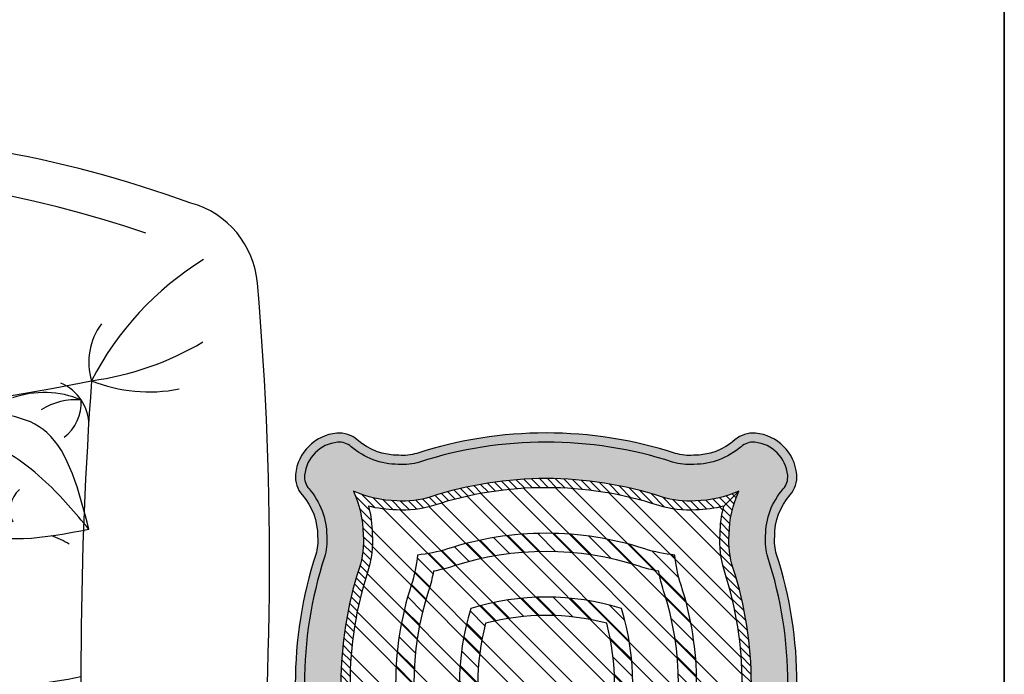
# Model space of a CAD drawing. Units: inches. Extents: x 844 to 2234, y 346 to 1084.
# Tile 41 of 93: x 1266.41 to 1283.62, y 719.22 to 730.66. Entities that reach past the tile are written whole.
import ezdxf

# ---------------------------------------------------------------- set-up
doc = ezdxf.new("R2010")
doc.units = ezdxf.units.IN
doc.header["$MEASUREMENT"] = 0
doc.layers.add('A-WALL', color=7, linetype='Continuous', lineweight=35)
doc.layers.add('furniture', color=8, linetype='Continuous', lineweight=18)
for name, color, linetype in [('RA-AP-01$0$FURN', 3, 'Continuous'), ('RA-AP-01$0$steel', 193, 'Continuous'), ('RA-AP-01$0$WOOD', 64, 'Continuous')]:
    doc.layers.add(name, color=color, linetype=linetype)
pattern_1 = [(45, (0, 1.362436106329781), (-0.0088388347648318, 0.0088388347648318), [])]
pattern_2 = [(45, (0, 1.362436106329781), (-0.0044194173824159, 0.0044194173824159), [])]

# ---------------------------------------------------------------- blocks, each defined once
blk = doc.blocks.new('A$C2FCF5309')
at = {"layer": 'RA-AP-01$0$FURN'}
h = blk.add_hatch(dxfattribs=at)
h.set_pattern_fill('ANSI31', color=256, scale=0.1, style=0)
h.set_pattern_definition(pattern_1)
h.paths.add_polyline_path([(5.038683893313746, -5.169250834004607, -0.1583983521602212), (5.038683893312098, -5.373464580902012, 0.0306258898943267), (5.033304057242972, -5.394827569605182, 0.0306258898948892), (5.01194106853941, -5.40020740567441, -0.1028142994996694), (4.878286182323899, -5.414871334512708), (4.863600873530158, -5.43331743520547, 0.1120482678681049), (5.018059823131753, -5.419248541734471, -0.052642197802937), (5.050972078299936, -5.412495590662115, -0.0526421977994963), (5.057725029371615, -5.379583335496025, 0.1583028414702701), (5.057725029372958, -5.163132079409654, -0.052642197806903), (5.050972078299777, -5.130219824239078, -0.0526421977995126), (5.018059823133679, -5.123466873167369, 0.0215995840215353), (4.988903013548211, -5.115372132362452), (4.975007495303644, -5.132826183367946, -0.0289147572844802), (5.011941068537408, -5.142508009226167, 0.0306258898976746), (5.033304057242868, -5.147887845296027, 0.0306258899022411)])
h.paths.add_polyline_path([(4.975007495303645, -5.132826183367946), (4.988903013548211, -5.115372132362452, 0.1362374241599938), (4.801608567045604, -5.12346687316654, -0.0526421978036853), (4.768696311876971, -5.130219824239102, -0.05264219780204), (4.761943360804856, -5.163132079406747, 0.1583028414743723), (4.761943360806116, -5.379583335498449, -0.0526421977955461), (4.768696311877141, -5.412495590662114, -0.0526421978073986), (4.801608567048022, -5.419248541735437, 0.0454484293938888), (4.863600873530158, -5.43331743520547), (4.878286182323899, -5.414871334512708, -0.0546933379798044), (4.80772732164382, -5.40020740567649, 0.030625889903973), (4.786364332934043, -5.394827569605216, 0.0306258898932853), (4.780984496865101, -5.373464580902791, -0.1583983521638281), (4.780984496864308, -5.169250834000963, 0.03062588989692), (4.786364332933943, -5.147887845296004, 0.0306258898946324), (4.807727321637318, -5.142508009226805, -0.1288932573266927)])
h.paths.add_polyline_path([(4.843422214712861, -5.204945727074827, -0.0783685831716868), (4.924134454130224, -5.196727409635105), (4.939146578618322, -5.177870798323143, 0.1012675676854134), (4.827248748758957, -5.188772261120899, 0.1253648873081696), (4.820394258584192, -5.327034652050361), (4.837127701354095, -5.306015906404253, -0.0981593964869636)], flags=17)
h.paths.add_polyline_path([(4.843422214712824, -5.337769687826355, -0.0311091841722656), (4.837127701354095, -5.306015906404253), (4.820394258584193, -5.32703465205036, 0.0247727657431944), (4.827248748758908, -5.353943153780261, 0.0812754385032542), (4.916962478476905, -5.36629034358622), (4.933684093813825, -5.345286454285511, -0.0876255421014372)], flags=17)
h.paths.add_polyline_path([(4.992419641418037, -5.353943153780226, 0.1506053783834298), (4.992419641417933, -5.188772261120954, 0.0485966419124224), (4.939146578618321, -5.177870798323143), (4.924134454130224, -5.196727409635105, -0.0507799419579301), (4.976246175464031, -5.204945727074882, -0.1296645318906876), (4.97624617546411, -5.337769687826316, -0.0415667119298777), (4.933684093813825, -5.345286454285511), (4.916962478476905, -5.36629034358622, 0.0684915676023693)], flags=17)
h = blk.add_hatch(dxfattribs=at)
h.set_pattern_fill('ANSI31', color=256, scale=0.1, style=0)
h.set_pattern_definition(pattern_1)
h.paths.add_polyline_path([(5.038683893313746, -5.169250834004607, -0.1583983521602212), (5.038683893312098, -5.373464580902012, 0.0306258898943267), (5.033304057242972, -5.394827569605182, 0.0306258898948892), (5.01194106853941, -5.40020740567441, -0.1028142994996694), (4.878286182323899, -5.414871334512708), (4.863600873530158, -5.43331743520547, 0.1120482678681049), (5.018059823131753, -5.419248541734471, -0.052642197802937), (5.050972078299936, -5.412495590662115, -0.0526421977994963), (5.057725029371615, -5.379583335496025, 0.1583028414702701), (5.057725029372958, -5.163132079409654, -0.052642197806903), (5.050972078299777, -5.130219824239078, -0.0526421977995126), (5.018059823133679, -5.123466873167369, 0.0215995840215353), (4.988903013548211, -5.115372132362452), (4.975007495303644, -5.132826183367946, -0.0289147572844802), (5.011941068537408, -5.142508009226167, 0.0306258898976746), (5.033304057242868, -5.147887845296027, 0.0306258899022411)])
h.paths.add_polyline_path([(4.975007495303645, -5.132826183367946), (4.988903013548211, -5.115372132362452, 0.1362374241599938), (4.801608567045604, -5.12346687316654, -0.0526421978036853), (4.768696311876971, -5.130219824239102, -0.05264219780204), (4.761943360804856, -5.163132079406747, 0.1583028414743723), (4.761943360806116, -5.379583335498449, -0.0526421977955461), (4.768696311877141, -5.412495590662114, -0.0526421978073986), (4.801608567048022, -5.419248541735437, 0.0454484293938888), (4.863600873530158, -5.43331743520547), (4.878286182323899, -5.414871334512708, -0.0546933379798044), (4.80772732164382, -5.40020740567649, 0.030625889903973), (4.786364332934043, -5.394827569605216, 0.0306258898932853), (4.780984496865101, -5.373464580902791, -0.1583983521638281), (4.780984496864308, -5.169250834000963, 0.03062588989692), (4.786364332933943, -5.147887845296004, 0.0306258898946324), (4.807727321637318, -5.142508009226805, -0.1288932573266927)])
h.paths.add_polyline_path([(4.843422214712861, -5.204945727074827, -0.0783685831716868), (4.924134454130224, -5.196727409635105), (4.939146578618322, -5.177870798323143, 0.1012675676854134), (4.827248748758957, -5.188772261120899, 0.1253648873081696), (4.820394258584192, -5.327034652050361), (4.837127701354095, -5.306015906404253, -0.0981593964869636)], flags=17)
h.paths.add_polyline_path([(4.843422214712824, -5.337769687826355, -0.0311091841722656), (4.837127701354095, -5.306015906404253), (4.820394258584193, -5.32703465205036, 0.0247727657431944), (4.827248748758908, -5.353943153780261, 0.0812754385032542), (4.916962478476905, -5.36629034358622), (4.933684093813825, -5.345286454285511, -0.0876255421014372)], flags=17)
h.paths.add_polyline_path([(4.992419641418037, -5.353943153780226, 0.1506053783834298), (4.992419641417933, -5.188772261120954, 0.0485966419124224), (4.939146578618321, -5.177870798323143), (4.924134454130224, -5.196727409635105, -0.0507799419579301), (4.976246175464031, -5.204945727074882, -0.1296645318906876), (4.97624617546411, -5.337769687826316, -0.0415667119298777), (4.933684093813825, -5.345286454285511), (4.916962478476905, -5.36629034358622, 0.0684915676023693)], flags=17)
at = {"layer": 'RA-AP-01$0$WOOD'}
h = blk.add_hatch(color=256, dxfattribs=at)
edge = h.paths.add_edge_path()
edge.add_arc((4.683001772622394, -5.026441828662609), 0.0299999999999998, 48.77105092035535, 95.25687599427813)
edge.add_arc((4.684834195088484, -5.046357707450686), 0.0499999999998897, 95.25687599443106, 174.7431240064049)
edge.add_arc((4.664918316300367, -5.044525284985046), 0.0300000000000005, 174.7431240062535, 221.2289490796905)
edge.add_arc((4.591236830209155, -5.109094338216345), 0.0679700159630267, -0.5333070513215148, 41.228949079691915, ccw=False)
edge.add_arc((4.609451302807284, -5.114694777173187), 0.0500000000000008, -17.3556839752095, 5.7020707654044145, ccw=False)
edge.add_arc((5.095208119646659, -5.271357707450659), 0.4603971832811796, 162.0683908477609, 197.9316091523306)
edge.add_arc((4.609451302807533, -5.428020637728902), 0.0500000000000006, -5.702070765320514, 17.355683975293914, ccw=False)
edge.add_arc((4.591236830209412, -5.433621076685779), 0.0679700159630261, -41.228949079600625, 0.5333070514128053, ccw=False)
edge.add_arc((4.664918316300727, -5.498190129916959), 0.0299999999999995, 138.7710509204022, 185.256875994324)
edge.add_arc((4.684834195088642, -5.496357707450695), 0.0499999999997451, 185.2568759946742, 264.74312400432)
edge.add_arc((4.683001772622394, -5.516273586238612), 0.03, 264.743124003969, 311.2289490796446)
edge.add_arc((4.747570825853633, -5.589955072329876), 0.0679700159630271, 89.4666929486321, 131.2289490796457, ccw=False)
edge.add_arc((4.753171264810493, -5.57174059973175), 0.0500000000000015, 72.64431602474701, 95.70207076536133, ccw=False)
edge.add_arc((4.909834195088355, -5.085983782892503), 0.4603971832811774, 252.0683908477147, 287.9316091522845)
edge.add_arc((5.06649712536621, -5.57174059973175), 0.0499999999999999, 84.29792923463953, 107.35568397525361, ccw=False)
edge.add_arc((5.072097564323069, -5.589955072329877), 0.0679700159630274, 48.771050920354185, 90.5333070513679, ccw=False)
edge.add_arc((5.136666617554309, -5.516273586238614), 0.0299999999999997, 228.771050920353, 275.2568759942969)
edge.add_arc((5.134834195088338, -5.496357707450417), 0.0499999999999982, 275.2568759942949, 354.7431240057633)
edge.add_arc((5.154750073876535, -5.498190129916372), 0.0299999999999999, 354.7431240057662, 401.2289490796891)
edge.add_arc((5.228431559967749, -5.433621076685074), 0.0679700159630274, 179.4666929486771, 221.2289490796903, ccw=False)
edge.add_arc((5.210217087369615, -5.428020637728227), 0.0499999999999976, 162.6443160247947, 185.7020707654089, ccw=False)
edge.add_arc((4.724460270530244, -5.271357707450757), 0.4603971832811793, 342.0683908477607, 377.9316091523305)
edge.add_arc((5.210217087369368, -5.114694777172509), 0.0500000000000019, 174.2979292346878, 197.355683975302, ccw=False)
edge.add_arc((5.228431559967489, -5.109094338215639), 0.0679700159630279, 138.7710509203993, 180.5333070514128, ccw=False)
edge.add_arc((5.154750073876174, -5.044525284984457), 0.0300000000000001, 318.771050920401, 365.2568759954636)
edge.add_arc((5.13483419508816, -5.046357707450624), 0.0499999999998349, 5.256875995237118, 84.74312400549572)
edge.add_arc((5.136666617554308, -5.026441828662608), 0.0299999999999994, 84.74312400572185, 131.2289490796446)
edge.add_arc((5.072097564323072, -4.952760342571343), 0.0679700159630261, 269.4666929486298, 311.22894907964354, ccw=False)
edge.add_arc((5.066497125366206, -4.97097481516947), 0.0499999999999992, 252.64431602475162, 275.70207076536565, ccw=False)
edge.add_arc((4.909834195088355, -5.456731632008717), 0.4603971832811764, 72.06839084771546, 107.9316091522853)
edge.add_arc((4.753171264810493, -4.970974815169471), 0.0500000000000016, 264.2979292346387, 287.355683975253, ccw=False)
edge.add_arc((4.747570825853633, -4.952760342571346), 0.0679700159630274, 228.7710509203543, 270.5333070513679, ccw=False)
edge = h.paths.add_edge_path(flags=16)
edge.add_arc((4.683001772622395, -5.026441828662608), 0.019999999999999, 48.7710509203555, 95.2568759942793)
edge.add_arc((4.684834195088469, -5.046357707450671), 0.0399999999998731, 95.2568759944489, 174.7431240064248)
edge.add_arc((4.664918316300404, -5.044525284985035), 0.020000000000036, 174.7431240062186, 221.2289490796461)
edge.add_arc((4.591236830209151, -5.109094338216346), 0.0779700159630296, -0.13764630038667747, 41.228949079689585, ccw=False)
edge.add_arc((4.609451302807307, -5.11469477717304), 0.060000000000024, -17.406127045137907, 5.176192161068002, ccw=False)
edge.add_arc((5.09520811964665, -5.271357707450659), 0.4503971832811708, 162.0623235129628, 197.9376764869162)
edge.add_arc((4.609451302807532, -5.428020637728943), 0.0599999999999982, -5.176192160466428, 17.406127046715312, ccw=False)
edge.add_arc((4.591236830209414, -5.433621076685778), 0.0779700159630257, -41.2289490796029, 0.13764630095249686, ccw=False)
edge.add_arc((4.664918316300731, -5.498190129916961), 0.0200000000000047, 138.7710509204103, 185.2568759943212)
edge.add_arc((4.684834195088606, -5.496357707450731), 0.0399999999997066, 185.2568759947174, 264.7431240043665)
edge.add_arc((4.683001772622369, -5.516273586238541), 0.020000000000069, 264.7431240038842, 311.2289490795622)
edge.add_arc((4.747570825853635, -5.589955072329884), 0.0779700159630344, 89.8623536987642, 131.2289490796432, ccw=False)
edge.add_arc((4.753171264810603, -5.571740599731771), 0.0599999999999895, 72.5938729544394, 95.1761921602253, ccw=False)
edge.add_arc((4.909834195088365, -5.085983782892505), 0.4503971832811724, 252.0623235129989, 287.9376764870498)
edge.add_arc((5.066497125366216, -5.571740599731755), 0.0600000000000047, 84.8238078399923, 107.40612704528041, ccw=False)
edge.add_arc((5.072097564322998, -5.589955072329853), 0.077970015963056, 48.771050920303594, 90.13764630126451, ccw=False)
edge.add_arc((5.136666617554307, -5.516273586238622), 0.0199999999999931, 228.771050920344, 275.2568759943037)
edge.add_arc((5.134834195088338, -5.496357707450416), 0.0400000000000004, 275.2568759942928, 354.7431240057607)
edge.add_arc((5.154750073876533, -5.498190129916375), 0.0200000000000037, 354.7431240057783, 401.2289490796939)
edge.add_arc((5.228431559967745, -5.433621076685076), 0.0779700159630239, 179.8623536995147, 221.2289490796908, ccw=False)
edge.add_arc((5.210217087369586, -5.428020637728345), 0.0600000000000054, 162.5938729554486, 185.1761921609759, ccw=False)
edge.add_arc((4.724460270530243, -5.271357707450766), 0.4503971832811826, 342.0623235128896, 377.937676486982)
edge.add_arc((5.210217087369347, -5.114694777172486), 0.0599999999999777, 174.8238078387611, 197.4061270462219, ccw=False)
edge.add_arc((5.228431559967523, -5.109094338215542), 0.0779700159629885, 138.7710509204687, 180.1376463004423, ccw=False)
edge.add_arc((5.154750073876175, -5.044525284984459), 0.0199999999999989, 318.771050920406, 365.2568759954698)
edge.add_arc((5.134834195088138, -5.046357707450646), 0.0399999999998586, 5.256875995208452, 84.74312400546732)
edge.add_arc((5.136666617554292, -5.02644182866256), 0.0199999999999529, 84.74312400577769, 131.2289490797025)
edge.add_arc((5.072097564323069, -4.952760342571338), 0.077970015963032, 269.86235369901414, 311.2289490796421, ccw=False)
edge.add_arc((5.06649712536618, -4.97097481516946), 0.0600000000000007, 252.5938729548277, 275.17619216047467, ccw=False)
edge.add_arc((4.909834195088353, -5.456731632008716), 0.4503971832811739, 72.06232351293887, 107.9376764867365)
edge.add_arc((4.753171264810429, -4.970974815169467), 0.0599999999999991, 264.82380783985815, 287.40612704769893, ccw=False)
edge.add_arc((4.747570825853681, -4.952760342571361), 0.0779700159630467, 228.7710509203206, 270.13764630113724, ccw=False)
h = blk.add_hatch(color=256, dxfattribs=at)
edge = h.paths.add_edge_path()
edge.add_arc((4.683001772622395, -5.026441828662608), 0.019999999999999, 48.7710509203555, 95.2568759942793)
edge.add_arc((4.684834195088469, -5.046357707450671), 0.0399999999998731, 95.2568759944489, 174.7431240064248)
edge.add_arc((4.664918316300404, -5.044525284985035), 0.020000000000036, 174.7431240062186, 221.2289490796461)
edge.add_arc((4.591236830209151, -5.109094338216346), 0.0779700159630296, -0.13764630038667747, 41.228949079689585, ccw=False)
edge.add_arc((4.609451302807307, -5.11469477717304), 0.060000000000024, -17.406127045137907, 5.176192161068002, ccw=False)
edge.add_arc((5.09520811964665, -5.271357707450659), 0.4503971832811708, 162.0623235129628, 197.9376764869162)
edge.add_arc((4.609451302807532, -5.428020637728943), 0.0599999999999982, -5.176192160466428, 17.406127046715312, ccw=False)
edge.add_arc((4.591236830209414, -5.433621076685778), 0.0779700159630257, -41.2289490796029, 0.13764630095249686, ccw=False)
edge.add_arc((4.664918316300731, -5.498190129916961), 0.0200000000000047, 138.7710509204103, 185.2568759943212)
edge.add_arc((4.684834195088606, -5.496357707450731), 0.0399999999997066, 185.2568759947174, 264.7431240043665)
edge.add_arc((4.683001772622369, -5.516273586238541), 0.020000000000069, 264.7431240038842, 311.2289490795622)
edge.add_arc((4.747570825853635, -5.589955072329884), 0.0779700159630344, 89.8623536987642, 131.2289490796432, ccw=False)
edge.add_arc((4.753171264810603, -5.571740599731771), 0.0599999999999895, 72.5938729544394, 95.1761921602253, ccw=False)
edge.add_arc((4.909834195088365, -5.085983782892505), 0.4503971832811724, 252.0623235129989, 287.9376764870498)
edge.add_arc((5.066497125366216, -5.571740599731755), 0.0600000000000047, 84.8238078399923, 107.40612704528041, ccw=False)
edge.add_arc((5.072097564322998, -5.589955072329853), 0.077970015963056, 48.771050920303594, 90.13764630126451, ccw=False)
edge.add_arc((5.136666617554307, -5.516273586238622), 0.0199999999999931, 228.771050920344, 275.2568759943037)
edge.add_arc((5.134834195088338, -5.496357707450416), 0.0400000000000004, 275.2568759942928, 354.7431240057607)
edge.add_arc((5.154750073876533, -5.498190129916375), 0.0200000000000037, 354.7431240057783, 401.2289490796939)
edge.add_arc((5.228431559967745, -5.433621076685076), 0.0779700159630239, 179.8623536995147, 221.2289490796908, ccw=False)
edge.add_arc((5.210217087369586, -5.428020637728345), 0.0600000000000054, 162.5938729554486, 185.1761921609759, ccw=False)
edge.add_arc((4.724460270530243, -5.271357707450766), 0.4503971832811826, 342.0623235128896, 377.937676486982)
edge.add_arc((5.210217087369347, -5.114694777172486), 0.0599999999999777, 174.8238078387611, 197.4061270462219, ccw=False)
edge.add_arc((5.228431559967523, -5.109094338215542), 0.0779700159629885, 138.7710509204687, 180.1376463004423, ccw=False)
edge.add_arc((5.154750073876175, -5.044525284984459), 0.0199999999999989, 318.771050920406, 365.2568759954698)
edge.add_arc((5.134834195088138, -5.046357707450646), 0.0399999999998586, 5.256875995208452, 84.74312400546732)
edge.add_arc((5.136666617554292, -5.02644182866256), 0.0199999999999529, 84.74312400577769, 131.2289490797025)
edge.add_arc((5.072097564323069, -4.952760342571338), 0.077970015963032, 269.86235369901414, 311.2289490796421, ccw=False)
edge.add_arc((5.06649712536618, -4.97097481516946), 0.0600000000000007, 252.5938729548277, 275.17619216047467, ccw=False)
edge.add_arc((4.909834195088353, -5.456731632008716), 0.4503971832811739, 72.06232351293887, 107.9376764867365)
edge.add_arc((4.753171264810429, -4.970974815169467), 0.0599999999999991, 264.82380783985815, 287.40612704769893, ccw=False)
edge.add_arc((4.747570825853681, -4.952760342571361), 0.0779700159630467, 228.7710509203206, 270.13764630113724, ccw=False)
edge = h.paths.add_edge_path(flags=16)
edge.add_arc((4.591236830209151, -5.109094338216348), 0.1179700159630308, 0.7417751874182841, 24.563326950263672, ccw=False)
edge.add_arc((4.609451302807302, -5.114694777173093), 0.100000000000012, -17.52836504564658, 4.087328884225087, ccw=False)
edge.add_arc((5.095208119646651, -5.271357707450657), 0.4103971832811724, 162.0403002448777, 197.9596997550675)
edge.add_arc((4.60945130280753, -5.428020637728918), 0.1000000000000027, -4.087328883827581, 17.528365046291924, ccw=False)
edge.add_arc((4.591236830209414, -5.433621076685779), 0.1179700159630246, 335.43667305041845, 359.2582248129738, ccw=False)
edge.add_arc((4.747570825853596, -5.589955072329891), 0.117970015963042, 90.7417751868461, 114.5633269496104, ccw=False)
edge.add_arc((4.753171264810559, -5.571740599731767), 0.0999999999999976, 72.47163495370341, 94.0873288836737, ccw=False)
edge.add_arc((4.909834195088367, -5.085983782892503), 0.4103971832811735, 252.0403002449999, 287.9596997551833)
edge.add_arc((5.066497125366205, -5.571740599731755), 0.1000000000000057, 85.91267111645209, 107.5283650455624, ccw=False)
edge.add_arc((5.072097564322985, -5.58995507232986), 0.117970015963046, 65.4366730497672, 89.25822481317113, ccw=False)
edge.add_arc((5.22843155996773, -5.433621076684992), 0.1179700159630096, 180.7417751873964, 204.5633269502712, ccw=False)
edge.add_arc((5.210217087369591, -5.428020637728301), 0.0999999999999969, 162.4716349546276, 184.0873288841682, ccw=False)
edge.add_arc((4.724460270530243, -5.271357707450766), 0.4103971832811825, 342.0403002448147, 377.9596997550345)
edge.add_arc((5.210217087369347, -5.114694777172489), 0.0999999999999796, 175.9126711156995, 197.5283650464392, ccw=False)
edge.add_arc((5.228431559967512, -5.109094338215525), 0.1179700159630019, 155.4366730502992, 179.2582248126247, ccw=False)
edge.add_arc((5.072097564323172, -4.952760342571314), 0.1179700159630537, 270.74177518697286, 294.56332694975765, ccw=False)
edge.add_arc((5.066497125366189, -4.970974815169462), 0.1000000000000017, 252.471634954247, 274.0873288838353, ccw=False)
edge.add_arc((4.909834195088353, -5.456731632008716), 0.4103971832811758, 72.04030024486342, 107.9596997549354)
edge.add_arc((4.75317126481046, -4.970974815169467), 0.1000000000000041, 265.91267111635307, 287.5283650466103, ccw=False)
edge.add_arc((4.747570825853629, -4.952760342571342), 0.1179700159630538, 245.43667304992562, 269.2582248131125, ccw=False)
h = blk.add_hatch(dxfattribs=at)
h.set_pattern_fill('ANSI31', color=256, scale=0.05, style=0)
h.set_pattern_definition(pattern_2)
h.paths.add_polyline_path([(5.105336294329346, -5.394854099602528, 0.0940138826956367), (5.100476366643778, -5.435568764288975, 0.0606271852326483), (5.104678567100611, -5.466202079462671, 0.0606271852344644), (5.074045251925975, -5.46199987900586, 0.0940138827021426), (5.033330587236848, -5.466859806692645, -0.1305325492494615), (4.828072633169377, -5.477944178050054), (4.821119726105699, -5.486677669841435, 0.1336226599878005), (5.036379334063467, -5.476383803188216, -0.0945969211935747), (5.073624810952389, -5.471994942692536, -0.1043170707892296), (5.121137550891356, -5.48266106325342, -0.1043170707868944), (5.110471430330457, -5.435148323315565, -0.0945969211952573), (5.114860290825935, -5.397902846425963, 0.1580239521433527), (5.114860290826324, -5.144812568476775, -0.0945969212010491), (5.110471430330247, -5.10756709158498, -0.1043170707844371), (5.121137550890657, -5.060054351648168, -0.104317070786514), (5.073624810952866, -5.070720472208642, -0.0945969211958523), (5.036379334063063, -5.066331611712874, 0.1580239521426795), (4.783289056114906, -5.066331611712465, -0.0945969211985319), (4.746043579224103, -5.070720472208672, -0.1043170707882665), (4.698530839285552, -5.060054351647925, -0.1043170707867205), (4.709196959846443, -5.10756709158571, -0.094596921196788), (4.704808099350826, -5.144812568475902, 0.1580239521433127), (4.704808099350699, -5.397902846425022, -0.094596921197841), (4.709196959846712, -5.435148323315576, -0.1043170707855109), (4.698530839286393, -5.482661063252921, -0.1043170707864168), (4.746043579224162, -5.471994942692571, -0.0945969211977586), (4.783289056114671, -5.476383803188671, 0.0238966994662183), (4.821119726105699, -5.486677669841435), (4.828072633169378, -5.477944178050054, -0.0269814195959459), (4.786337802940177, -5.466859806692736, 0.0940138827039629), (4.745623138250268, -5.461999879005895, 0.0606271852320776), (4.714989823076826, -5.466202079462476, 0.0606271852304618), (4.719192023533341, -5.435568764289856, 0.0940138826917763), (4.714332095848404, -5.394854099604977, -0.1580706864542086), (4.714332095846561, -5.147861315302034, 0.0940138827032017), (4.719192023533127, -5.107146650612438, 0.0606271852329446), (4.714989823076289, -5.076513335438588, 0.0606271852340035), (4.745623138250698, -5.08071553589536, 0.0940138827025969), (4.786337802940015, -5.075855608208526, -0.1580706864508517), (5.033330587237968, -5.075855608208939, 0.0940138827009578), (5.074045251926627, -5.080715535895319, 0.0606271852322557), (5.104678567100159, -5.076513335438697, 0.0606271852308743), (5.100476366643561, -5.107146650611519, 0.0940138827178109), (5.105336294331983, -5.147861315307182, -0.1580706864490946)])
h = blk.add_hatch(dxfattribs=at)
h.set_pattern_fill('ANSI31', color=256, scale=0.05, style=0)
h.set_pattern_definition(pattern_2)
h.paths.add_polyline_path([(5.105336294329346, -5.394854099602528, 0.0940138826956367), (5.100476366643778, -5.435568764288975, 0.0606271852326483), (5.104678567100611, -5.466202079462671, 0.0606271852344644), (5.074045251925975, -5.46199987900586, 0.0940138827021426), (5.033330587236848, -5.466859806692645, -0.1305325492494615), (4.828072633169377, -5.477944178050054), (4.821119726105699, -5.486677669841435, 0.1336226599878005), (5.036379334063467, -5.476383803188216, -0.0945969211935747), (5.073624810952389, -5.471994942692536, -0.1043170707892296), (5.121137550891356, -5.48266106325342, -0.1043170707868944), (5.110471430330457, -5.435148323315565, -0.0945969211952573), (5.114860290825935, -5.397902846425963, 0.1580239521433527), (5.114860290826324, -5.144812568476775, -0.0945969212010491), (5.110471430330247, -5.10756709158498, -0.1043170707844371), (5.121137550890657, -5.060054351648168, -0.104317070786514), (5.073624810952866, -5.070720472208642, -0.0945969211958523), (5.036379334063063, -5.066331611712874, 0.1580239521426795), (4.783289056114906, -5.066331611712465, -0.0945969211985319), (4.746043579224103, -5.070720472208672, -0.1043170707882665), (4.698530839285552, -5.060054351647925, -0.1043170707867205), (4.709196959846443, -5.10756709158571, -0.094596921196788), (4.704808099350826, -5.144812568475902, 0.1580239521433127), (4.704808099350699, -5.397902846425022, -0.094596921197841), (4.709196959846712, -5.435148323315576, -0.1043170707855109), (4.698530839286393, -5.482661063252921, -0.1043170707864168), (4.746043579224162, -5.471994942692571, -0.0945969211977586), (4.783289056114671, -5.476383803188671, 0.0238966994662183), (4.821119726105699, -5.486677669841435), (4.828072633169378, -5.477944178050054, -0.0269814195959459), (4.786337802940177, -5.466859806692736, 0.0940138827039629), (4.745623138250268, -5.461999879005895, 0.0606271852320776), (4.714989823076826, -5.466202079462476, 0.0606271852304618), (4.719192023533341, -5.435568764289856, 0.0940138826917763), (4.714332095848404, -5.394854099604977, -0.1580706864542086), (4.714332095846561, -5.147861315302034, 0.0940138827032017), (4.719192023533127, -5.107146650612438, 0.0606271852329446), (4.714989823076289, -5.076513335438588, 0.0606271852340035), (4.745623138250698, -5.08071553589536, 0.0940138827025969), (4.786337802940015, -5.075855608208526, -0.1580706864508517), (5.033330587237968, -5.075855608208939, 0.0940138827009578), (5.074045251926627, -5.080715535895319, 0.0606271852322557), (5.104678567100159, -5.076513335438697, 0.0606271852308743), (5.100476366643561, -5.107146650611519, 0.0940138827178109), (5.105336294331983, -5.147861315307182, -0.1580706864490946)])
h = blk.add_hatch(dxfattribs=at)
h.set_pattern_fill('ANSI32,_I', color=256, scale=0.1, style=2)
h.set_pattern_definition([(45, (0, 0), (-0.0265165042944955, 0.0265165042944955), []), (45, (0.0176776695, 0), (-0.0265165042944955, 0.0265165042944955), [])])
h.paths.add_polyline_path([(4.843422214712824, -5.337769687826354, 0.1296645318905289), (4.97624617546411, -5.337769687826316, 0.1296645318906876), (4.976246175464032, -5.204945727074882, 0.129664531890418), (4.843422214712861, -5.204945727074827, 0.129664531890765)], flags=0)
h.paths.add_polyline_path([(5.039131224122924, -5.170637849998464, -0.0326520429852175), (5.033304057242868, -5.147887845296027, -0.0326520429894721), (5.010554052537512, -5.142060678415043, 0.1561383235202698), (4.809114337641437, -5.142060678414318, -0.0326520429925972), (4.786364332933944, -5.147887845296004, -0.0326520429914489), (4.780537166052582, -5.170637850002729, 0.1561383235189577), (4.780537166052134, -5.37207756489719, -0.0326520429934175), (4.786364332934042, -5.394827569605215, -0.0326520429823496), (4.809114337634529, -5.400654736484653, 0.156138323524066), (5.010554052535268, -5.400654736486903, -0.032652042992888), (5.033304057242972, -5.394827569605183, -0.0326520429928733), (5.039131224124712, -5.372077564897496, 0.1561383235226786)], flags=0)
h.paths.add_polyline_path([(4.992419641418037, -5.353943153780226, -0.1506053783832862), (4.827248748758909, -5.353943153780261, -0.1506053783835069), (4.827248748758957, -5.188772261120899, -0.1506053783831346), (4.992419641417933, -5.188772261120954, -0.1506053783834298)], flags=0)
h.paths.add_polyline_path([(4.976246175464111, -5.337769687826316, -0.1296645318905298), (4.843422214712824, -5.337769687826354, -0.129664531890765), (4.843422214712862, -5.204945727074827, -0.1296645318904162), (4.976246175464031, -5.204945727074882, -0.1296645318906876)], flags=0)
h.paths.add_polyline_path([(5.105721254232479, -5.149054940982025, -0.0968902512052664), (5.100476366643561, -5.107146650611519, -0.0606271852308743), (5.104678567100159, -5.076513335438697, -0.0606271852322574), (5.074045251926626, -5.080715535895319, -0.0968902512197216), (5.032136961550132, -5.075470648304253, 0.1564657949319774), (4.787531428625239, -5.075470648304682, -0.0968902512150626), (4.745623138250699, -5.08071553589536, -0.060627185234009), (4.714989823076288, -5.076513335438587, -0.0606271852329501), (4.719192023533127, -5.10714665061244, -0.0968902512185585), (4.713947135942331, -5.149054940988458, 0.1564657949285579), (4.713947135940853, -5.393660473908259, -0.0968902512319826), (4.71919202353334, -5.435568764289873, -0.0606271852304288), (4.714989823076825, -5.466202079462476, -0.0606271852320811), (4.745623138250269, -5.461999879005895, -0.0968902512162649), (4.787531428625332, -5.467244766596559, 0.1564657949327057), (5.032136961551311, -5.46724476659659, -0.0968902512153659), (5.074045251925975, -5.46199987900586, -0.0606271852344627), (5.10467856710061, -5.466202079462671, -0.0606271852326483), (5.100476366643777, -5.435568764288975, -0.0968902512258216), (5.105721254235559, -5.393660473909953, 0.1564657949340142)])
h.paths.add_polyline_path([(5.057725029371625, -5.379583335495999, 0.0526421977995391), (5.050972078299936, -5.412495590662114, 0.0526421978029782), (5.018059823131728, -5.419248541734479, -0.1583028414681072), (4.801608567048168, -5.419248541735485, 0.0526421978076402), (4.76869631187714, -5.412495590662113, 0.0526421977956189), (4.761943360806101, -5.379583335498404, -0.1583028414743129), (4.761943360804846, -5.163132079406778, 0.0526421978020944), (4.768696311876972, -5.130219824239101, 0.0526421978033651), (4.80160856704541, -5.123466873166602, -0.1583028414716875), (5.018059823133628, -5.123466873167353, 0.0526421977995944), (5.050972078299776, -5.130219824239078, 0.0526421978070423), (5.057725029372986, -5.163132079409739, -0.1583028414701848)], flags=16)
h.paths.add_polyline_path([(5.038683893312112, -5.373464580901968, 0.0306258898943915), (5.033304057242972, -5.394827569605182, 0.0306258898948892), (5.01194106853941, -5.40020740567441, -0.1583983521587032), (4.807727321643864, -5.400207405676503, 0.0306258899040366), (4.786364332934043, -5.394827569605215, 0.0306258898931986), (4.780984496865119, -5.37346458090285, -0.1583983521638542), (4.7809844968643, -5.169250834000989, 0.0306258898969596), (4.786364332933945, -5.147887845296004, 0.0306258898946195), (4.807727321637311, -5.142508009226808, -0.1583983521623412), (5.011941068537318, -5.142508009226139, 0.030625889897807), (5.033304057242868, -5.147887845296028, 0.0306258899020632), (5.038683893313706, -5.169250834004486, -0.1583983521602835)], flags=0)
for p, q in [((4.714989823076289, -5.076513335438588), (4.698530839285552, -5.060054351647925)), ((4.714989823076289, -5.076513335438588), (4.698530839285552, -5.060054351647925)), ((5.104678567100159, -5.076513335438697), (5.121137550890656, -5.060054351648169)), ((5.104678567100159, -5.076513335438697), (5.121137550890656, -5.060054351648169)), ((5.10467856710061, -5.466202079462671), (5.121137550891355, -5.482661063253419)), ((5.10467856710061, -5.466202079462671), (5.121137550891355, -5.482661063253419))]:
    blk.add_line(p, q, dxfattribs=at)
for points in [[(4.702773858784635, -5.003879368495489, 0.2056608120285223), (4.680253138923443, -4.996568010480312, 0.3614336704708569), (4.635044498118043, -5.041776651286372, 0.2056608120263112), (4.642355856133262, -5.064297371147306, -0.1842662638101064), (4.65920390179375, -5.10972699154053, -0.1009492694051416), (4.657174869772992, -5.129609908955028, 0.1577727036674954), (4.657174869773219, -5.41310550594699, -0.1009492694051416), (4.659203901794006, -5.432988423361486, -0.1842662638101064), (4.64235585613359, -5.478418043754737, 0.2056608120285221), (4.635044498118431, -5.500938763615934, 0.3614336704593693), (4.680253138922529, -5.546147404420826, 0.2056608120364936), (4.702773858784635, -5.538836046405732, -0.1842662638101064), (4.748203479177874, -5.52198800074528, -0.1009492694051415), (4.768086396592371, -5.524017032766053, 0.1577727036674954), (5.051581993584332, -5.524017032766055, -0.1009492694051416), (5.071464910998829, -5.521988000745282, -0.1842662638101064), (5.116894531392067, -5.538836046405734, 0.2056608120286145), (5.13941525125327, -5.546147404420911, 0.3614336704683636), (5.184623892058835, -5.500938763615299, 0.2056608120285223), (5.177312534043641, -5.478418043754112, -0.1842662638101063), (5.160464488383153, -5.432988423360887, -0.1009492694051416), (5.162493520403909, -5.41310550594639, 0.1577727036674954), (5.162493520403684, -5.129609908954428, -0.1009492694051416), (5.160464488382894, -5.109726991539933, -0.1842662638101064), (5.17731253404331, -5.064297371146681, 0.2056608120337072), (5.184623892058415, -5.041776651284888, 0.3614336704623863), (5.139415251253259, -4.99656801048031, 0.2056608120285223), (5.116894531392067, -5.003879368495487, -0.1842662638101064), (5.071464910998829, -5.020727414155937, -0.1009492694051416), (5.051581993584332, -5.018698382135166, 0.1577727036674956), (4.768086396592371, -5.018698382135168, -0.1009492694051416), (4.748203479177874, -5.020727414155941, -0.1842662638101064)], [(4.702773858784635, -5.003879368495489, 0.2056608120285223), (4.680253138923443, -4.996568010480312, 0.3614336704708569), (4.635044498118043, -5.041776651286372, 0.2056608120263112), (4.642355856133262, -5.064297371147306, -0.1842662638101064), (4.65920390179375, -5.10972699154053, -0.1009492694051416), (4.657174869772992, -5.129609908955028, 0.1577727036674954), (4.657174869773219, -5.41310550594699, -0.1009492694051416), (4.659203901794006, -5.432988423361486, -0.1842662638101064), (4.64235585613359, -5.478418043754737, 0.2056608120285221), (4.635044498118431, -5.500938763615934, 0.3614336704593693), (4.680253138922529, -5.546147404420826, 0.2056608120364936), (4.702773858784635, -5.538836046405732, -0.1842662638101064), (4.748203479177874, -5.52198800074528, -0.1009492694051415), (4.768086396592371, -5.524017032766053, 0.1577727036674954), (5.051581993584332, -5.524017032766055, -0.1009492694051416), (5.071464910998829, -5.521988000745282, -0.1842662638101064), (5.116894531392067, -5.538836046405734, 0.2056608120286145), (5.13941525125327, -5.546147404420911, 0.3614336704683636), (5.184623892058835, -5.500938763615299, 0.2056608120285223), (5.177312534043641, -5.478418043754112, -0.1842662638101063), (5.160464488383153, -5.432988423360887, -0.1009492694051416), (5.162493520403909, -5.41310550594639, 0.1577727036674954), (5.162493520403684, -5.129609908954428, -0.1009492694051416), (5.160464488382894, -5.109726991539933, -0.1842662638101064), (5.17731253404331, -5.064297371146681, 0.2056608120337072), (5.184623892058415, -5.041776651284888, 0.3614336704623863), (5.139415251253259, -4.99656801048031, 0.2056608120285223), (5.116894531392067, -5.003879368495487, -0.1842662638101064), (5.071464910998829, -5.020727414155937, -0.1009492694051416), (5.051581993584332, -5.018698382135166, 0.1577727036674956), (4.768086396592371, -5.018698382135168, -0.1009492694051416), (4.748203479177874, -5.020727414155941, -0.1842662638101064)], [(4.696183163397222, -5.011400188551196, 0.2056608120285295), (4.681169350156427, -5.006525949874411, 0.3614336704708588), (4.645002437512154, -5.042692862519237, 0.2056608120262659), (4.649876676188964, -5.057706675759887, -0.182481815856965), (4.669206621172843, -5.109281651732388, -0.0988540857970112), (4.666703803477437, -5.13264334722805, 0.1578269695851905), (4.666703803477144, -5.410072067672365, -0.0988540858013112), (4.6692066211731, -5.433433763168966, -0.1824818158591246), (4.649876676189301, -5.485008739142145, 0.2056608120284717), (4.64500243751253, -5.500022552382944, 0.3614336704593821), (4.681169350155757, -5.536189465026749, 0.2056608120365057), (4.696183163397221, -5.531315226350026, -0.1824818158605826), (4.747758139370833, -5.51198528136619, -0.0988540857951607), (4.771119834866025, -5.514488099061806, 0.1578269695856264), (5.04854855531107, -5.514488099061688, -0.0988540857929677), (5.071910250805761, -5.511985281366138, -0.1824818158609529), (5.123485226779481, -5.531315226350027, 0.2056608120286893), (5.138499040020282, -5.536189465026812, 0.3614336704683556), (5.174665952664737, -5.500022552382323, 0.2056608120284882), (5.169791713987938, -5.485008739141532, -0.1824818158574124), (5.150461769004059, -5.4334337631689, -0.0988540857940221), (5.152964586699289, -5.410072067673927, 0.1578269695858123), (5.1529645866996, -5.132643347228565, -0.0988540858025403), (5.150461769003872, -5.109281651731659, -0.1824818158565006), (5.169791713987599, -5.057706675759273, 0.2056608120337192), (5.174665952664335, -5.042692862518078, 0.3614336704623903), (5.138499040020236, -5.006525949874406, 0.2056608120285323), (5.123485226779481, -5.011400188551195, -0.1824818158594503), (5.071910250806212, -5.03073013353503, -0.09885408579455), (5.048548555311143, -5.028227315839558, 0.1578269695844942), (4.771119834867991, -5.028227315838772, -0.0988540858042156), (4.747758139370745, -5.030730133535067, -0.1824818158603032)], [(4.696183163397222, -5.011400188551196, 0.2056608120285295), (4.681169350156427, -5.006525949874411, 0.3614336704708588), (4.645002437512154, -5.042692862519237, 0.2056608120262659), (4.649876676188964, -5.057706675759887, -0.182481815856965), (4.669206621172843, -5.109281651732388, -0.0988540857970112), (4.666703803477437, -5.13264334722805, 0.1578269695851905), (4.666703803477144, -5.410072067672365, -0.0988540858013112), (4.6692066211731, -5.433433763168966, -0.1824818158591246), (4.649876676189301, -5.485008739142145, 0.2056608120284717), (4.64500243751253, -5.500022552382944, 0.3614336704593821), (4.681169350155757, -5.536189465026749, 0.2056608120365057), (4.696183163397221, -5.531315226350026, -0.1824818158605826), (4.747758139370833, -5.51198528136619, -0.0988540857951607), (4.771119834866025, -5.514488099061806, 0.1578269695856264), (5.04854855531107, -5.514488099061688, -0.0988540857929677), (5.071910250805761, -5.511985281366138, -0.1824818158609529), (5.123485226779481, -5.531315226350027, 0.2056608120286893), (5.138499040020282, -5.536189465026812, 0.3614336704683556), (5.174665952664737, -5.500022552382323, 0.2056608120284882), (5.169791713987938, -5.485008739141532, -0.1824818158574124), (5.150461769004059, -5.4334337631689, -0.0988540857940221), (5.152964586699289, -5.410072067673927, 0.1578269695858123), (5.1529645866996, -5.132643347228565, -0.0988540858025403), (5.150461769003872, -5.109281651731659, -0.1824818158565006), (5.169791713987599, -5.057706675759273, 0.2056608120337192), (5.174665952664335, -5.042692862518078, 0.3614336704623903), (5.138499040020236, -5.006525949874406, 0.2056608120285323), (5.123485226779481, -5.011400188551195, -0.1824818158594503), (5.071910250806212, -5.03073013353503, -0.09885408579455), (5.048548555311143, -5.028227315839558, 0.1578269695844942), (4.771119834867991, -5.028227315838772, -0.0988540858042156), (4.747758139370745, -5.030730133535067, -0.1824818158603032)], [(4.698530839285552, -5.060054351647925, -0.1043170707867612), (4.709196959846444, -5.107567091585729, -0.0945969211969405), (4.704808099350802, -5.144812568475978, 0.1580239521432241), (4.704808099350681, -5.397902846424963, -0.0945969211980322), (4.709196959846711, -5.43514832331559, -0.104317070785482), (4.698530839286393, -5.482661063252921, -0.1043170707864036), (4.746043579224155, -5.471994942692571, -0.094596921197375), (4.78328905611452, -5.476383803188623, 0.1580239521431959), (5.036379334063463, -5.476383803188218, -0.0945969211935888), (5.07362481095239, -5.471994942692536, -0.1043170707892253), (5.121137550891355, -5.482661063253419, -0.1043170707868921), (5.110471430330457, -5.435148323315565, -0.0945969211954828), (5.114860290825962, -5.397902846425878, 0.158023952143358), (5.114860290826295, -5.144812568476682, -0.0945969212007617), (5.110471430330247, -5.107567091584995, -0.1043170707844689), (5.121137550890656, -5.060054351648169, -0.1043170707864946), (5.073624810952874, -5.070720472208642, -0.0945969211956941), (5.036379334063131, -5.066331611712896, 0.1580239521426976), (4.783289056114946, -5.066331611712452, -0.0945969211986379), (4.746043579224103, -5.070720472208672, -0.1043170707882684)], [(4.698530839285552, -5.060054351647925, -0.1043170707867612), (4.709196959846444, -5.107567091585729, -0.0945969211969405), (4.704808099350802, -5.144812568475978, 0.1580239521432241), (4.704808099350681, -5.397902846424963, -0.0945969211980322), (4.709196959846711, -5.43514832331559, -0.104317070785482), (4.698530839286393, -5.482661063252921, -0.1043170707864036), (4.746043579224155, -5.471994942692571, -0.094596921197375), (4.78328905611452, -5.476383803188623, 0.1580239521431959), (5.036379334063463, -5.476383803188218, -0.0945969211935888), (5.07362481095239, -5.471994942692536, -0.1043170707892253), (5.121137550891355, -5.482661063253419, -0.1043170707868921), (5.110471430330457, -5.435148323315565, -0.0945969211954828), (5.114860290825962, -5.397902846425878, 0.158023952143358), (5.114860290826295, -5.144812568476682, -0.0945969212007617), (5.110471430330247, -5.107567091584995, -0.1043170707844689), (5.121137550890656, -5.060054351648169, -0.1043170707864946), (5.073624810952874, -5.070720472208642, -0.0945969211956941), (5.036379334063131, -5.066331611712896, 0.1580239521426976), (4.783289056114946, -5.066331611712452, -0.0945969211986379), (4.746043579224103, -5.070720472208672, -0.1043170707882684)], [(4.714989823076289, -5.076513335438588, -0.0606271852329464), (4.719192023533127, -5.107146650612439, -0.0940138827030756), (4.714332095846578, -5.147861315301983, 0.1580706864542707), (4.714332095848417, -5.394854099605018, -0.0940138826916965), (4.719192023533341, -5.435568764289864, -0.0606271852304462), (4.714989823076826, -5.466202079462476, -0.0606271852320585), (4.745623138250258, -5.461999879005895, -0.0940138827037036), (4.786337802940059, -5.466859806692699, 0.1580706864500221), (5.033330587236783, -5.466859806692666, -0.0940138827023111), (5.074045251925979, -5.46199987900586, -0.060627185234454), (5.10467856710061, -5.466202079462671, -0.0606271852326709), (5.100476366643777, -5.435568764288963, -0.0940138826958686), (5.105336294329379, -5.394854099602421, 0.1580706864489859), (5.105336294331999, -5.147861315307237, -0.0940138827179432), (5.100476366643561, -5.107146650611518, -0.0606271852308726), (5.104678567100159, -5.076513335438697, -0.0606271852322592), (5.074045251926625, -5.080715535895319, -0.094013882701022), (5.03333058723794, -5.075855608208931, 0.1580706864508015), (4.786337802940061, -5.075855608208511, -0.0940138827027143), (4.745623138250695, -5.08071553589536, -0.0606271852339983)], [(4.714989823076289, -5.076513335438588, -0.0606271852329464), (4.719192023533127, -5.107146650612439, -0.0940138827030756), (4.714332095846578, -5.147861315301983, 0.1580706864542707), (4.714332095848417, -5.394854099605018, -0.0940138826916965), (4.719192023533341, -5.435568764289864, -0.0606271852304462), (4.714989823076826, -5.466202079462476, -0.0606271852320585), (4.745623138250258, -5.461999879005895, -0.0940138827037036), (4.786337802940059, -5.466859806692699, 0.1580706864500221), (5.033330587236783, -5.466859806692666, -0.0940138827023111), (5.074045251925979, -5.46199987900586, -0.060627185234454), (5.10467856710061, -5.466202079462671, -0.0606271852326709), (5.100476366643777, -5.435568764288963, -0.0940138826958686), (5.105336294329379, -5.394854099602421, 0.1580706864489859), (5.105336294331999, -5.147861315307237, -0.0940138827179432), (5.100476366643561, -5.107146650611518, -0.0606271852308726), (5.104678567100159, -5.076513335438697, -0.0606271852322592), (5.074045251926625, -5.080715535895319, -0.094013882701022), (5.03333058723794, -5.075855608208931, 0.1580706864508015), (4.786337802940061, -5.075855608208511, -0.0940138827027143), (4.745623138250695, -5.08071553589536, -0.0606271852339983)], [(4.768696311876972, -5.130219824239102, -0.0526421978019087), (4.761943360804882, -5.163132079406667, 0.1583028414744761), (4.761943360806133, -5.379583335498504, -0.0526421977954539), (4.76869631187714, -5.412495590662113, -0.0526421978076619), (4.801608567048181, -5.419248541735488, 0.1583028414681522), (5.0180598231318, -5.419248541734456, -0.0526421978028585), (5.050972078299936, -5.412495590662114, -0.0526421977992923), (5.057725029371576, -5.379583335496149, 0.1583028414703719), (5.057725029372956, -5.163132079409646, -0.0526421978068888), (5.050972078299776, -5.130219824239078, -0.052642197799403), (5.018059823133745, -5.12346687316739, 0.1583028414717216), (4.801608567045482, -5.123466873166579, -0.0526421978034837)], [(4.768696311876972, -5.130219824239102, -0.0526421978019087), (4.761943360804882, -5.163132079406667, 0.1583028414744761), (4.761943360806133, -5.379583335498504, -0.0526421977954539), (4.76869631187714, -5.412495590662113, -0.0526421978076619), (4.801608567048181, -5.419248541735488, 0.1583028414681522), (5.0180598231318, -5.419248541734456, -0.0526421978028585), (5.050972078299936, -5.412495590662114, -0.0526421977992923), (5.057725029371576, -5.379583335496149, 0.1583028414703719), (5.057725029372956, -5.163132079409646, -0.0526421978068888), (5.050972078299776, -5.130219824239078, -0.052642197799403), (5.018059823133745, -5.12346687316739, 0.1583028414717216), (4.801608567045482, -5.123466873166579, -0.0526421978034837)], [(4.786364332933944, -5.147887845296004, -0.0306258898969254), (4.780984496864308, -5.169250834000966, 0.1583983521638412), (4.780984496865107, -5.373464580902811, -0.0306258898932568), (4.786364332934043, -5.394827569605216, -0.0306258899041339), (4.80772732164393, -5.400207405676526, 0.1583983521586416), (5.011941068539401, -5.400207405674413, -0.0306258898949021), (5.033304057242972, -5.394827569605182, -0.0306258898943513), (5.038683893312104, -5.373464580901996, 0.1583983521602784), (5.038683893313717, -5.16925083400452, -0.0306258899021139), (5.033304057242868, -5.147887845296027, -0.030625889897777), (5.011941068537338, -5.142508009226145, 0.1583983521624288), (4.807727321637224, -5.142508009226835, -0.0306258898944937)], [(4.786364332933944, -5.147887845296004, -0.0306258898969254), (4.780984496864308, -5.169250834000966, 0.1583983521638412), (4.780984496865107, -5.373464580902811, -0.0306258898932568), (4.786364332934043, -5.394827569605216, -0.0306258899041339), (4.80772732164393, -5.400207405676526, 0.1583983521586416), (5.011941068539401, -5.400207405674413, -0.0306258898949021), (5.033304057242972, -5.394827569605182, -0.0306258898943513), (5.038683893312104, -5.373464580901996, 0.1583983521602784), (5.038683893313717, -5.16925083400452, -0.0306258899021139), (5.033304057242868, -5.147887845296027, -0.030625889897777), (5.011941068537338, -5.142508009226145, 0.1583983521624288), (4.807727321637224, -5.142508009226835, -0.0306258898944937)], [(4.827248748758957, -5.1887722611209, 0.1506053783835061), (4.827248748758908, -5.353943153780261, 0.150605378383287), (4.992419641418037, -5.353943153780226, 0.1506053783834298), (4.992419641417933, -5.188772261120954, 0.1506053783831346)], [(4.827248748758957, -5.1887722611209, 0.1506053783835061), (4.827248748758908, -5.353943153780261, 0.150605378383287), (4.992419641418037, -5.353943153780226, 0.1506053783834298), (4.992419641417933, -5.188772261120954, 0.1506053783831346)], [(4.843422214712861, -5.204945727074827, 0.1296645318907659), (4.843422214712824, -5.337769687826355, 0.1296645318905299), (4.976246175464111, -5.337769687826316, 0.1296645318906876), (4.976246175464032, -5.204945727074882, 0.129664531890418)], [(4.843422214712861, -5.204945727074827, 0.1296645318907659), (4.843422214712824, -5.337769687826355, 0.1296645318905299), (4.976246175464111, -5.337769687826316, 0.1296645318906876), (4.976246175464032, -5.204945727074882, 0.129664531890418)]]:
    blk.add_lwpolyline(points, format="xyb", close=True, dxfattribs=at)
blk = doc.blocks.new('A$C7F4351E2')
at = {"layer": 'RA-AP-01$0$FURN'}
for p, q in [((8.352559572600457, -8.263941955512525), (8.35255957259913, -8.282283310927069)), ((8.352559572600457, -8.927748273106442), (8.35255957259913, -8.909406917691898))]:
    blk.add_line(p, q, dxfattribs=at)
at = {"layer": 'RA-AP-01$0$FURN', "const_width": 0.01}
for points in [[(8.437812509519787, -8.415359762755768, 1), (8.427812509519786, -8.415359762755742, 1)], [(8.758197489244363, -8.415359762756214, -1), (8.768197489244365, -8.415359762756214, -1)], [(8.437812509519787, -8.776330465863198, -1), (8.427812509519786, -8.776330465863225, -1)], [(8.758197489244363, -8.776330465862753, 1), (8.768197489244365, -8.776330465862753, 1)]]:
    blk.add_lwpolyline(points, format="xyb", close=True, dxfattribs=at)
at = {"layer": 'RA-AP-01$0$FURN'}
for centre, radius, start, end in [((8.727559572604601, -11.61690445537682), 3.552808610866049, 85.0473312316413, 96.05887237565803), ((8.50205957259015, -8.17394195551301), 0.1744999999876311, 148.9517780040467, 211.048221995953), ((9.025650106946005, -8.176987401637472), 0.1, 15.499494600857, 85.04733123164159), ((8.77247054904813, -7.958543863781743), 0.3382138395168437, 297.2303327094027, 328.2563708342649), ((9.2484631175852, -8.302692737637487), 0.3241573581843151, 149.2985674842688, 172.3026350986055), ((7.88981694267423, -8.595845114309485), 1.310286319972027, 340.1192502251003, 19.8807497748998), ((9.084915705374858, -8.196040134964925), 0.1698955038956699, 168.877843135945, 201.8512383801196), ((7.929864357850293, -8.595845114309483), 1.224941341589781, 341.1257460634955, 18.87425393650447), ((8.947672844970796, -8.191835192646359), 0.0704710051510922, 253.1338634205325, 306.4126496157095), ((8.408522229993444, -8.33300072568355), 0.0753785023123622, 115.8745619060558, 163.9833547230034), ((8.603635103111959, -3.79706073025477), 4.473931917517753, 266.7828902523826, 274.1477233631118), ((8.878389979098333, -8.312202545234353), 0.05, 30.14777190425723, 89.99999999905349), ((10.52713941284929, -8.595845114309466), 1.634931324962266, 168.1200364254424, 191.8799635745573), ((9.101231010340802, -8.38034106221356), 0.5100538472773755, 167.6182489359307, 193.3122231353938), ((8.903279781571525, -8.31837865610295), 0.0478550828899777, 86.575295631534, 142.6833829238214), ((8.838100984994732, -8.276822957859652), 0.0683206773889159, 326.6729861493449, 5.218395042636973), ((8.810121490949696, -8.31110757721543), 0.1042084262671507, 340.4828318717155, 22.86929393278168), ((8.395364730619693, -8.304213854581548), 0.0479292786975047, 152.8070868543555, 225.4025460716553), ((8.333592787569726, -8.402663469525104), 0.1218651776285568, 48.0375529564433, 81.04623209541253), ((7.439612310514541, -8.913795367824825), 1.11020813118073, 31.93286085977143, 34.66647731879807), ((8.553131949433, -8.344109762755968), 0.1214118203512435, 150.1419074485596, 187.691663289156), ((8.642878049331348, -8.344109762756093), 0.1214118203512435, 352.3083367106845, 29.85809255128089), ((9.82633505008426, -8.696671375220811), 1.539060359583382, 165.5338783218257, 176.2437734318419), ((8.374918524725835, -8.294321202996931), 0.1212957045587361, 247.3375839744822, 273.7314750942433), ((8.546954810732721, -8.753394424755975), 0.3517162425384579, 83.41248966761125, 103.1674570565571), ((8.697701155637269, -8.172468128267624), 0.2442261434243043, 248.9017070735605, 275.9923925191661), ((8.73287643248165, -8.469775898206471), 0.3023568492824586, 173.0944825511667, 197.588060785551), ((8.889871101981017, -8.492307869305423), 0.1295083186917369, 167.9901339202812, 211.3796151021958), ((8.444145567704187, -7.829943385268752), 0.765467899454341, 258.6273206109321, 281.4174148186357), ((8.781211457338294, -7.772561243483908), 0.8232838708255751, 260.2449188973366, 277.7495311655964), ((9.82633505008426, -8.495018853398156), 1.539060359583382, 183.7562265681581, 194.4661216781742), ((8.444145567704187, -9.361312955433425), 0.765467899454341, 78.58258518136427, 101.3726793890678), ((8.781211457338294, -9.418695097218269), 0.8232838708255751, 82.25060502413102, 99.75508110266344), ((8.73287643248165, -8.721914330412496), 0.3023568492824586, 162.411939214449, 186.9055174488332), ((8.889871101981017, -8.699382359313544), 0.1295083186917369, 148.6203848978042, 192.0098660797188), ((9.101231010340802, -8.811349166405407), 0.5100538472773755, 166.6877768646062, 192.3817510640693), ((8.799643412436344, -8.749969313933361), 0.0689028341546707, 265.5384273543114, 353.5804828909086), ((8.374918524725835, -8.897369025622035), 0.1212957045587361, 86.26852490575668, 112.6624160255178), ((8.697701155637269, -9.019222100351342), 0.2442261434243043, 84.00760748083387, 111.0982929264395), ((8.546954810732721, -8.438295803862992), 0.3517162425384579, 256.8325429434429, 276.5875103323888), ((8.553131949433, -8.847580465862999), 0.1214118203512435, 172.308336710844, 209.8580925514404), ((8.785133372574222, -8.874256642962408), 0.0310151388417235, 42.62105484496073, 114.2239681486109), ((8.810121490949696, -8.880582651403534), 0.1042084262671507, 337.1307060672183, 19.51716812828453), ((8.395364730619693, -8.88747637403742), 0.0479292786975047, 134.5974539283447, 207.1929131456445), ((7.439612310514541, -8.277894860794142), 1.11020813118073, 325.333522681202, 328.0671391402286), ((8.408522229993444, -8.858689502935416), 0.0753785023123622, 196.0166452769965, 244.1254380939442), ((8.333592787569726, -8.789026759093863), 0.1218651776285568, 278.9537679045875, 311.9624470435567), ((8.838100984994732, -8.914867270759315), 0.0683206773889159, 354.781604957363, 33.32701385065517), ((8.642878049331348, -8.847580465862874), 0.1214118203512435, 330.1419074487191, 340.3913536181062), ((8.903279781571525, -8.873311572516016), 0.0478550828899777, 217.3166170761785, 273.424704368466), ((8.878389979098333, -8.879487683384612), 0.05, 270.0000000009465, 337.4173275753961), ((8.50205957259015, -9.017748273105955), 0.1744999999876311, 148.9517780040469, 211.0482219959533), ((8.603635103111959, -13.39462949836419), 4.473931917517753, 85.85227663688822, 93.21710974761734), ((9.084915705374858, -8.995650093654042), 0.1698955038956699, 158.1487616198804, 191.122156864055), ((8.947672844970796, -8.999855035972608), 0.0704710051510922, 53.58735038429053, 106.8661365794674), ((8.77247054904813, -9.233146364837223), 0.3382138395168437, 31.74362916573515, 62.76966729059727), ((9.2484631175852, -8.88899749098148), 0.3241573581843151, 187.6973649013944, 210.7014325157311), ((9.025650106946005, -9.014702826981493), 0.1, 274.9526687683584, 344.500505399143), ((8.727559572604601, -5.574785773242145), 3.552808610866049, 263.941127624342, 274.9526687683587)]:
    blk.add_arc(centre, radius, start, end, dxfattribs=at)
for points, knots in [([(8.764421239581775, -8.929562504990262), (8.755250524728652, -8.881106864374377), (8.74196437992213, -8.810906376383404), (8.80604948961138, -8.740469753734786), (8.847474678848357, -8.701097198289744), (8.897142214037096, -8.58322730303861), (8.897091569728207, -8.784804210134517), (8.88612504526093, -8.897825917224484), (8.806539053396843, -8.9185794820093), (8.764421239581775, -8.92956250499026)], [0, 0, 0, 0, 0.1367586589314792, 0.1981301758052368, 0.2677729570689282, 0.3281194902553322, 0.4737578340741565, 0.5765194025309516, 0.6920332287422236, 0.6920332287422236, 0.6920332287422236, 0.6920332287422236]), ([(8.764421239581775, -8.92956250499026), (8.782204778269502, -8.914603263160053), (8.821592007255505, -8.881471326160916), (8.86917941606436, -8.814322636989944), (8.867818990542759, -8.729338202119969), (8.881231406199264, -8.676770566934765), (8.888101821971249, -8.649843164808122)], [0, 0, 0, 0, 0.070018540671015, 0.1550780383534498, 0.2344491945777043, 0.3178048737568289, 0.3178048737568289, 0.3178048737568289, 0.3178048737568289])]:
    blk.add_open_spline(points, degree=3, knots=knots, dxfattribs=at)
blk = doc.blocks.new('A$C5D2F253E')
at = {"layer": 'RA-AP-01$0$steel', "xscale": -1}
blk.add_blockref('A$C2FCF5309', (6.339960502260055, 7.248884637679282), dxfattribs=at)
at = {"layer": 'RA-AP-01$0$WOOD', "xscale": -1, "rotation": 180}
blk.add_blockref('A$C7F4351E2', (-7.164808785335935, -7.45332973198748), dxfattribs=at)

msp = doc.modelspace()

# ---------------------------------------------------------------- linework, layer by layer
at = {"layer": 'A-WALL'}
msp.add_line((1283.615947594791, 761.3107742764157), (1283.615947594791, 624.3107742764157), dxfattribs=at)

# ---------------------------------------------------------------- block references
at = {"layer": 'furniture', "xscale": -15.94108302203742, "yscale": 15.94108302203742, "zscale": 15.94108302203742, "rotation": 270}
msp.add_blockref('A$C5D2F253E', (1244.08405109492, 696.2584716700112), dxfattribs=at)

doc.saveas('drawing.dxf')
